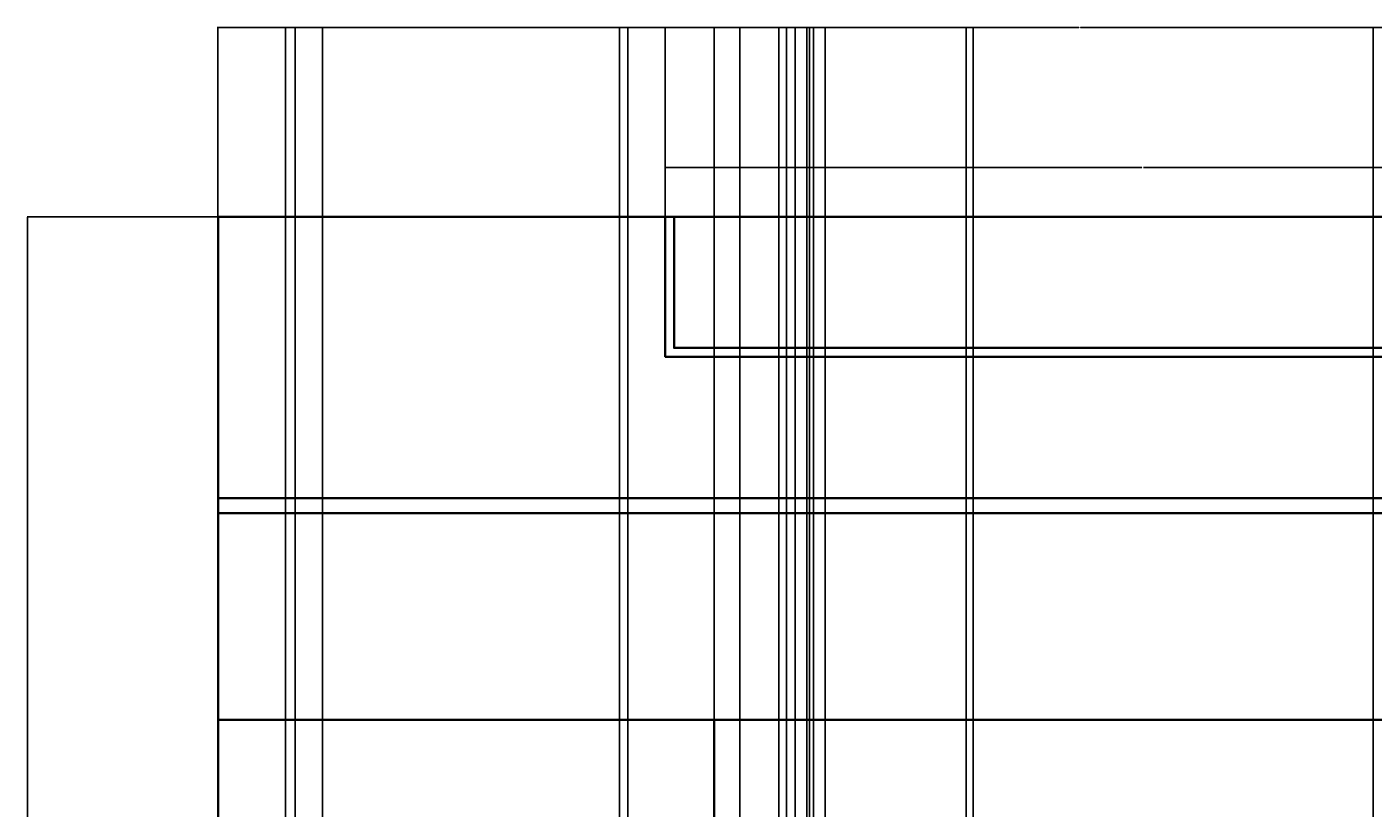
# Model space of a CAD drawing. Units: inches. Extents: x 1231 to 2151, y 481 to 2277.
# Tile 6 of 7: x 1231 to 1819, y 1935 to 2277. Entities that reach past the tile are written whole.
import ezdxf

# ---------------------------------------------------------------- set-up
doc = ezdxf.new("R2010")
doc.units = ezdxf.units.IN
doc.header["$MEASUREMENT"] = 0
doc.layers.add('A-ANNO-DIMS', color=2, linetype='Continuous', lineweight=18)
doc.layers.add('A-ELEV', color=7, linetype='Continuous', lineweight=35)
doc.styles.get("Standard").update_dxf_attribs({"font": 'arial.ttf'})
doc.dimstyles.get("Standard").update_dxf_attribs({"dimtxt": 0.18, "dimasz": 0.18, "dimexe": 0.18, "dimexo": 0.0625, "dimgap": 0.09, "dimtad": 0, "dimtih": 1, "dimtoh": 1, "dimdec": 0, "dimzin": 0, "dimdsep": 46, "dimlunit": 3, "dimtxsty": 'Standard', "dimcen": 0.09, "dimadec": 0, "dimazin": 0, "dimtfac": 1, "dimtdec": 0, "dimtofl": 0, "dimtmove": 0, "dimatfit": 3, "dimfxl": 1, "dimtolj": 1, "dimtzin": 0, "dimarcsym": 0})

# ---------------------------------------------------------------- blocks, each defined once
blk = doc.blocks.new('*D2')
at = {"layer": 'A-ANNO-DIMS', "color": 0, "lineweight": -2, "transparency": 16777216}
for p, q in [((1314.18, 2193.78), (1230.78, 2193.78)), ((1230.96, 2193.6), (1230.96, 1378.92)), ((1230.96, 563.87), (1230.96, 1378.55)), ((1314.18, 563.69), (1230.78, 563.69))]:
    blk.add_line(p, q, dxfattribs=at)
at = {"layer": 'A-ANNO-DIMS', "color": 0, "transparency": 16777216}
for points in [[(1230.93, 2193.6), (1230.99, 2193.6), (1230.96, 2193.78)], [(1230.93, 563.87), (1230.99, 563.87), (1230.96, 563.69)]]:
    blk.add_solid(points, dxfattribs=at)
at = {"layer": 'Defpoints', "color": 0, "transparency": 16777216}
for p in [(1230.96, 2193.78), (1314.24, 2193.78), (1314.24, 563.69)]:
    blk.add_point(p, dxfattribs=at)
at = {"layer": 'A-ANNO-DIMS', "color": 0, "transparency": 16777216, "insert": (1230.96, 1378.74), "char_height": 0.18, "attachment_point": 5}
blk.add_mtext('\\A1;1630', dxfattribs=at)
blk = doc.blocks.new('*D15')
at = {"layer": 'A-ANNO-DIMS', "color": 0, "lineweight": -2, "transparency": 16777216}
for p, q in [((1314.24, 1475.61), (1314.24, 2276.71)), ((1314.42, 2276.53), (1328.56, 2276.53)), ((1343.64, 2276.53), (1329.49, 2276.53)), ((1343.82, 1512.24), (1343.82, 2276.71))]:
    blk.add_line(p, q, dxfattribs=at)
at = {"layer": 'A-ANNO-DIMS', "color": 0, "transparency": 16777216}
for points in [[(1314.42, 2276.56), (1314.42, 2276.5), (1314.24, 2276.53)], [(1343.64, 2276.56), (1343.64, 2276.5), (1343.82, 2276.53)]]:
    blk.add_solid(points, dxfattribs=at)
at = {"layer": 'Defpoints', "color": 0, "transparency": 16777216}
for p in [(1343.82, 2276.53), (1343.82, 1512.17), (1314.24, 1475.54)]:
    blk.add_point(p, dxfattribs=at)
at = {"layer": 'A-ANNO-DIMS', "color": 0, "transparency": 16777216, "insert": (1329.03, 2276.53), "char_height": 0.18, "attachment_point": 5}
blk.add_mtext('\\A1;29.575', dxfattribs=at)
blk = doc.blocks.new('*D16')
at = {"layer": 'A-ANNO-DIMS', "color": 0, "lineweight": -2, "transparency": 16777216}
for p, q in [((1343.82, 1512.24), (1343.82, 2276.71)), ((1344, 2276.53), (1418.14, 2276.53)), ((1493.2, 2276.53), (1419.06, 2276.53)), ((1493.38, 1512.24), (1493.38, 2276.71))]:
    blk.add_line(p, q, dxfattribs=at)
at = {"layer": 'A-ANNO-DIMS', "color": 0, "transparency": 16777216}
for points in [[(1344, 2276.56), (1344, 2276.5), (1343.82, 2276.53)], [(1493.2, 2276.56), (1493.2, 2276.5), (1493.38, 2276.53)]]:
    blk.add_solid(points, dxfattribs=at)
at = {"layer": 'Defpoints', "color": 0, "transparency": 16777216}
for p in [(1493.38, 2276.53), (1343.82, 1512.17), (1493.38, 1512.17)]:
    blk.add_point(p, dxfattribs=at)
at = {"layer": 'A-ANNO-DIMS', "color": 0, "transparency": 16777216, "insert": (1418.6, 2276.53), "char_height": 0.18, "attachment_point": 5}
blk.add_mtext('\\A1;149.57', dxfattribs=at)
blk = doc.blocks.new('*D17')
at = {"layer": 'A-ANNO-DIMS', "color": 0, "lineweight": -2, "transparency": 16777216}
for p, q in [((1493.38, 1512.24), (1493.38, 2276.71)), ((1493.56, 2276.53), (1527.71, 2276.53)), ((1562.61, 2276.53), (1528.46, 2276.53)), ((1562.79, 1475.61), (1562.79, 2276.71))]:
    blk.add_line(p, q, dxfattribs=at)
at = {"layer": 'A-ANNO-DIMS', "color": 0, "transparency": 16777216}
for points in [[(1493.56, 2276.56), (1493.56, 2276.5), (1493.38, 2276.53)], [(1562.61, 2276.56), (1562.61, 2276.5), (1562.79, 2276.53)]]:
    blk.add_solid(points, dxfattribs=at)
at = {"layer": 'Defpoints', "color": 0, "transparency": 16777216}
for p in [(1562.79, 2276.53), (1493.38, 1512.17), (1562.79, 1475.54)]:
    blk.add_point(p, dxfattribs=at)
at = {"layer": 'A-ANNO-DIMS', "color": 0, "transparency": 16777216, "insert": (1528.09, 2276.53), "char_height": 0.18, "attachment_point": 5}
blk.add_mtext('\\A1;69.41', dxfattribs=at)
blk = doc.blocks.new('*D18')
at = {"layer": 'A-ANNO-DIMS', "color": 0, "lineweight": -2, "transparency": 16777216}
for p, q in [((1562.79, 1914.62), (1562.79, 2276.71)), ((1562.97, 2276.53), (1690.65, 2276.53)), ((1819.13, 2276.53), (1691.45, 2276.53)), ((1819.31, 1914.62), (1819.31, 2276.71))]:
    blk.add_line(p, q, dxfattribs=at)
at = {"layer": 'A-ANNO-DIMS', "color": 0, "transparency": 16777216}
for points in [[(1562.97, 2276.56), (1562.97, 2276.5), (1562.79, 2276.53)], [(1819.13, 2276.56), (1819.13, 2276.5), (1819.31, 2276.53)]]:
    blk.add_solid(points, dxfattribs=at)
at = {"layer": 'Defpoints', "color": 0, "transparency": 16777216}
for p in [(1819.31, 2276.53), (1562.79, 1914.56), (1819.31, 1914.56)]:
    blk.add_point(p, dxfattribs=at)
at = {"layer": 'A-ANNO-DIMS', "color": 0, "transparency": 16777216, "insert": (1691.05, 2276.53), "char_height": 0.18, "attachment_point": 5}
blk.add_mtext('\\A1;256.5', dxfattribs=at)
blk = doc.blocks.new('*D22')
at = {"layer": 'A-ANNO-DIMS', "color": 0, "lineweight": -2, "transparency": 16777216}
for p, q in [((1314.24, 1973.95), (1314.24, 2276.71)), ((1314.42, 2276.53), (1422.26, 2276.53)), ((1531.03, 2276.53), (1423.19, 2276.53)), ((1531.21, 1973.95), (1531.21, 2276.71))]:
    blk.add_line(p, q, dxfattribs=at)
at = {"layer": 'A-ANNO-DIMS', "color": 0, "transparency": 16777216}
for points in [[(1314.42, 2276.56), (1314.42, 2276.5), (1314.24, 2276.53)], [(1531.03, 2276.56), (1531.03, 2276.5), (1531.21, 2276.53)]]:
    blk.add_solid(points, dxfattribs=at)
at = {"layer": 'Defpoints', "color": 0, "transparency": 16777216}
for p in [(1531.21, 2276.53), (1314.24, 1973.89), (1531.21, 1973.89)]:
    blk.add_point(p, dxfattribs=at)
at = {"layer": 'A-ANNO-DIMS', "color": 0, "transparency": 16777216, "insert": (1422.73, 2276.53), "char_height": 0.18, "attachment_point": 5}
blk.add_mtext('\\A1;216.97', dxfattribs=at)
blk = doc.blocks.new('*D23')
at = {"layer": 'A-ANNO-DIMS', "color": 0, "lineweight": -2, "transparency": 16777216}
for p, q in [((1531.21, 1973.95), (1531.21, 2276.71)), ((1531.39, 2276.53), (1690.57, 2276.53)), ((1850.54, 2276.53), (1691.36, 2276.53)), ((1850.72, 1973.95), (1850.72, 2276.71))]:
    blk.add_line(p, q, dxfattribs=at)
at = {"layer": 'A-ANNO-DIMS', "color": 0, "transparency": 16777216}
for points in [[(1531.39, 2276.56), (1531.39, 2276.5), (1531.21, 2276.53)], [(1850.54, 2276.56), (1850.54, 2276.5), (1850.72, 2276.53)]]:
    blk.add_solid(points, dxfattribs=at)
at = {"layer": 'Defpoints', "color": 0, "transparency": 16777216}
for p in [(1850.72, 2276.53), (1531.21, 1973.89), (1850.72, 1973.89)]:
    blk.add_point(p, dxfattribs=at)
at = {"layer": 'A-ANNO-DIMS', "color": 0, "transparency": 16777216, "insert": (1690.96, 2276.53), "char_height": 0.18, "attachment_point": 5}
blk.add_mtext('\\A1;319.5', dxfattribs=at)
blk = doc.blocks.new('*D25')
at = {"layer": 'A-ANNO-DIMS', "color": 0, "lineweight": -2, "transparency": 16777216}
for p, q in [((1314.24, 2193.84), (1314.24, 2276.71)), ((1314.42, 2276.53), (1411.56, 2276.53)), ((1509.61, 2276.53), (1412.47, 2276.53)), ((1509.79, 2193.84), (1509.79, 2276.71))]:
    blk.add_line(p, q, dxfattribs=at)
at = {"layer": 'A-ANNO-DIMS', "color": 0, "transparency": 16777216}
for points in [[(1314.42, 2276.56), (1314.42, 2276.5), (1314.24, 2276.53)], [(1509.61, 2276.56), (1509.61, 2276.5), (1509.79, 2276.53)]]:
    blk.add_solid(points, dxfattribs=at)
at = {"layer": 'Defpoints', "color": 0, "transparency": 16777216}
for p in [(1509.79, 2276.53), (1314.24, 2193.78), (1509.79, 2193.78)]:
    blk.add_point(p, dxfattribs=at)
at = {"layer": 'A-ANNO-DIMS', "color": 0, "transparency": 16777216, "insert": (1412.02, 2276.53), "char_height": 0.18, "attachment_point": 5}
blk.add_mtext('\\A1;195.55', dxfattribs=at)
blk = doc.blocks.new('*D26')
at = {"layer": 'A-ANNO-DIMS', "color": 0, "lineweight": -2, "transparency": 16777216}
for p, q in [((1509.79, 2132.61), (1509.79, 2215.48)), ((1509.97, 2215.3), (1718.14, 2215.3)), ((1927.1, 2215.3), (1718.93, 2215.3)), ((1927.28, 2132.61), (1927.28, 2215.48))]:
    blk.add_line(p, q, dxfattribs=at)
at = {"layer": 'A-ANNO-DIMS', "color": 0, "transparency": 16777216}
for points in [[(1509.97, 2215.33), (1509.97, 2215.27), (1509.79, 2215.3)], [(1927.1, 2215.33), (1927.1, 2215.27), (1927.28, 2215.3)]]:
    blk.add_solid(points, dxfattribs=at)
at = {"layer": 'Defpoints', "color": 0, "transparency": 16777216}
for p in [(1927.28, 2215.3), (1509.79, 2132.55), (1927.28, 2132.55)]:
    blk.add_point(p, dxfattribs=at)
at = {"layer": 'A-ANNO-DIMS', "color": 0, "transparency": 16777216, "insert": (1718.53, 2215.3), "char_height": 0.18, "attachment_point": 5}
blk.add_mtext('\\A1;417.5', dxfattribs=at)
blk = doc.blocks.new('*D32')
at = {"layer": 'A-ANNO-DIMS', "color": 0, "lineweight": -2, "transparency": 16777216}
for p, q in [((1314.24, 1043.75), (1314.24, 2276.71)), ((1314.42, 2276.53), (1336.68, 2276.53)), ((1359.73, 2276.53), (1337.47, 2276.53)), ((1359.91, 1037.75), (1359.91, 2276.71))]:
    blk.add_line(p, q, dxfattribs=at)
at = {"layer": 'A-ANNO-DIMS', "color": 0, "transparency": 16777216}
for points in [[(1314.42, 2276.56), (1314.42, 2276.5), (1314.24, 2276.53)], [(1359.73, 2276.56), (1359.73, 2276.5), (1359.91, 2276.53)]]:
    blk.add_solid(points, dxfattribs=at)
at = {"layer": 'Defpoints', "color": 0, "transparency": 16777216}
for p in [(1359.91, 2276.53), (1314.24, 1043.69), (1359.91, 1037.69)]:
    blk.add_point(p, dxfattribs=at)
at = {"layer": 'A-ANNO-DIMS', "color": 0, "transparency": 16777216, "insert": (1337.07, 2276.53), "char_height": 0.18, "attachment_point": 5}
blk.add_mtext('\\A1;45.67', dxfattribs=at)
blk = doc.blocks.new('*D33')
at = {"layer": 'A-ANNO-DIMS', "color": 0, "lineweight": -2, "transparency": 16777216}
for p, q in [((1359.91, 1037.75), (1359.91, 2276.71)), ((1360.09, 2276.53), (1424.43, 2276.53)), ((1489.68, 2276.53), (1425.34, 2276.53)), ((1489.86, 1037.75), (1489.86, 2276.71))]:
    blk.add_line(p, q, dxfattribs=at)
at = {"layer": 'A-ANNO-DIMS', "color": 0, "transparency": 16777216}
for points in [[(1360.09, 2276.56), (1360.09, 2276.5), (1359.91, 2276.53)], [(1489.68, 2276.56), (1489.68, 2276.5), (1489.86, 2276.53)]]:
    blk.add_solid(points, dxfattribs=at)
at = {"layer": 'Defpoints', "color": 0, "transparency": 16777216}
for p in [(1489.86, 2276.53), (1359.91, 1037.69), (1489.86, 1037.69)]:
    blk.add_point(p, dxfattribs=at)
at = {"layer": 'A-ANNO-DIMS', "color": 0, "transparency": 16777216, "insert": (1424.88, 2276.53), "char_height": 0.18, "attachment_point": 5}
blk.add_mtext('\\A1;129.95', dxfattribs=at)
blk = doc.blocks.new('*D34')
at = {"layer": 'A-ANNO-DIMS', "color": 0, "lineweight": -2, "transparency": 16777216}
for p, q in [((1489.86, 1037.75), (1489.86, 2276.71)), ((1490.04, 2276.53), (1515.72, 2276.53)), ((1542.2, 2276.53), (1516.51, 2276.53)), ((1542.38, 1043.75), (1542.38, 2276.71))]:
    blk.add_line(p, q, dxfattribs=at)
at = {"layer": 'A-ANNO-DIMS', "color": 0, "transparency": 16777216}
for points in [[(1490.04, 2276.56), (1490.04, 2276.5), (1489.86, 2276.53)], [(1542.2, 2276.56), (1542.2, 2276.5), (1542.38, 2276.53)]]:
    blk.add_solid(points, dxfattribs=at)
at = {"layer": 'Defpoints', "color": 0, "transparency": 16777216}
for p in [(1542.38, 2276.53), (1542.38, 1043.69), (1489.86, 1037.69)]:
    blk.add_point(p, dxfattribs=at)
at = {"layer": 'A-ANNO-DIMS', "color": 0, "transparency": 16777216, "insert": (1516.12, 2276.53), "char_height": 0.18, "attachment_point": 5}
blk.add_mtext('\\A1;52.52', dxfattribs=at)
blk = doc.blocks.new('*D35')
at = {"layer": 'A-ANNO-DIMS', "color": 0, "lineweight": -2, "transparency": 16777216}
for p, q in [((1542.38, 1043.75), (1542.38, 2276.71)), ((1542.56, 2276.53), (1556.6, 2276.53)), ((1571.58, 2276.53), (1557.53, 2276.53)), ((1571.76, 1043.75), (1571.76, 2276.71))]:
    blk.add_line(p, q, dxfattribs=at)
at = {"layer": 'A-ANNO-DIMS', "color": 0, "transparency": 16777216}
for points in [[(1542.56, 2276.56), (1542.56, 2276.5), (1542.38, 2276.53)], [(1571.58, 2276.56), (1571.58, 2276.5), (1571.76, 2276.53)]]:
    blk.add_solid(points, dxfattribs=at)
at = {"layer": 'Defpoints', "color": 0, "transparency": 16777216}
for p in [(1571.76, 2276.53), (1542.38, 1043.69), (1571.76, 1043.69)]:
    blk.add_point(p, dxfattribs=at)
at = {"layer": 'A-ANNO-DIMS', "color": 0, "transparency": 16777216, "insert": (1557.07, 2276.53), "char_height": 0.18, "attachment_point": 5}
blk.add_mtext('\\A1;29.385', dxfattribs=at)
blk = doc.blocks.new('*D36')
at = {"layer": 'A-ANNO-DIMS', "color": 0, "lineweight": -2, "transparency": 16777216}
for p, q in [((1571.76, 1043.75), (1571.76, 2276.71)), ((1571.94, 2276.53), (1575.38, 2276.53)), ((1579.61, 2276.53), (1576.17, 2276.53)), ((1579.79, 1032.87), (1579.79, 2276.71))]:
    blk.add_line(p, q, dxfattribs=at)
at = {"layer": 'A-ANNO-DIMS', "color": 0, "transparency": 16777216}
for points in [[(1571.94, 2276.56), (1571.94, 2276.5), (1571.76, 2276.53)], [(1579.61, 2276.56), (1579.61, 2276.5), (1579.79, 2276.53)]]:
    blk.add_solid(points, dxfattribs=at)
at = {"layer": 'Defpoints', "color": 0, "transparency": 16777216}
for p in [(1579.79, 2276.53), (1571.76, 1043.69), (1579.79, 1032.81)]:
    blk.add_point(p, dxfattribs=at)
at = {"layer": 'A-ANNO-DIMS', "color": 0, "transparency": 16777216, "insert": (1575.78, 2276.53), "char_height": 0.18, "attachment_point": 5}
blk.add_mtext('\\A1;8.033', dxfattribs=at)
blk = doc.blocks.new('*D50')
at = {"layer": 'A-ANNO-DIMS', "color": 0, "lineweight": -2, "transparency": 16777216}
for p, q in [((1542.38, 563.75), (1542.38, 2276.71)), ((1542.56, 2276.53), (1550.52, 2276.53)), ((1559.26, 2276.53), (1551.3, 2276.53)), ((1559.44, 576.65), (1559.44, 2276.71))]:
    blk.add_line(p, q, dxfattribs=at)
at = {"layer": 'A-ANNO-DIMS', "color": 0, "transparency": 16777216}
for points in [[(1542.56, 2276.56), (1542.56, 2276.5), (1542.38, 2276.53)], [(1559.26, 2276.56), (1559.26, 2276.5), (1559.44, 2276.53)]]:
    blk.add_solid(points, dxfattribs=at)
at = {"layer": 'Defpoints', "color": 0, "transparency": 16777216}
for p in [(1559.44, 2276.53), (1559.44, 576.59), (1542.38, 563.69)]:
    blk.add_point(p, dxfattribs=at)
at = {"layer": 'A-ANNO-DIMS', "color": 0, "transparency": 16777216, "insert": (1550.91, 2276.53), "char_height": 0.18, "attachment_point": 5}
blk.add_mtext('\\A1;17.07', dxfattribs=at)
blk = doc.blocks.new('*D58')
at = {"layer": 'A-ANNO-DIMS', "color": 0, "lineweight": -2, "transparency": 16777216}
for p, q in [((1314.24, 1475.61), (1314.24, 2276.71)), ((1314.42, 2276.53), (1330.74, 2276.53)), ((1347.85, 2276.53), (1331.53, 2276.53)), ((1348.03, 1451.84), (1348.03, 2276.71))]:
    blk.add_line(p, q, dxfattribs=at)
at = {"layer": 'A-ANNO-DIMS', "color": 0, "transparency": 16777216}
for points in [[(1314.42, 2276.56), (1314.42, 2276.5), (1314.24, 2276.53)], [(1347.85, 2276.56), (1347.85, 2276.5), (1348.03, 2276.53)]]:
    blk.add_solid(points, dxfattribs=at)
at = {"layer": 'Defpoints', "color": 0, "transparency": 16777216}
for p in [(1348.03, 2276.53), (1314.24, 1475.54), (1348.03, 1451.77)]:
    blk.add_point(p, dxfattribs=at)
at = {"layer": 'A-ANNO-DIMS', "color": 0, "transparency": 16777216, "insert": (1331.14, 2276.53), "char_height": 0.18, "attachment_point": 5}
blk.add_mtext('\\A1;33.79', dxfattribs=at)
blk = doc.blocks.new('*D94')
at = {"layer": 'A-ANNO-DIMS', "color": 0, "lineweight": -2, "transparency": 16777216}
for p, q in [((1566.56, 1479.38), (1566.56, 2276.71)), ((1566.74, 2276.53), (1570.19, 2276.53)), ((1574.42, 2276.53), (1570.98, 2276.53)), ((1574.6, 1494.2), (1574.6, 2276.71))]:
    blk.add_line(p, q, dxfattribs=at)
at = {"layer": 'A-ANNO-DIMS', "color": 0, "transparency": 16777216}
for points in [[(1566.74, 2276.56), (1566.74, 2276.5), (1566.56, 2276.53)], [(1574.42, 2276.56), (1574.42, 2276.5), (1574.6, 2276.53)]]:
    blk.add_solid(points, dxfattribs=at)
at = {"layer": 'Defpoints', "color": 0, "transparency": 16777216}
for p in [(1574.6, 2276.53), (1574.6, 1494.13), (1566.56, 1479.32)]:
    blk.add_point(p, dxfattribs=at)
at = {"layer": 'A-ANNO-DIMS', "color": 0, "transparency": 16777216, "insert": (1570.58, 2276.53), "char_height": 0.18, "attachment_point": 5}
blk.add_mtext('\\A1;8.042', dxfattribs=at)
blk = doc.blocks.new('*D95')
at = {"layer": 'A-ANNO-DIMS', "color": 0, "lineweight": -2, "transparency": 16777216}
for p, q in [((1574.6, 1494.2), (1574.6, 2276.71)), ((1574.78, 2276.53), (1607.58, 2276.53)), ((1641.16, 2276.53), (1608.37, 2276.53)), ((1641.34, 1494.2), (1641.34, 2276.71))]:
    blk.add_line(p, q, dxfattribs=at)
at = {"layer": 'A-ANNO-DIMS', "color": 0, "transparency": 16777216}
for points in [[(1574.78, 2276.56), (1574.78, 2276.5), (1574.6, 2276.53)], [(1641.16, 2276.56), (1641.16, 2276.5), (1641.34, 2276.53)]]:
    blk.add_solid(points, dxfattribs=at)
at = {"layer": 'Defpoints', "color": 0, "transparency": 16777216}
for p in [(1641.34, 2276.53), (1574.6, 1494.13), (1641.34, 1494.13)]:
    blk.add_point(p, dxfattribs=at)
at = {"layer": 'A-ANNO-DIMS', "color": 0, "transparency": 16777216, "insert": (1607.97, 2276.53), "char_height": 0.18, "attachment_point": 5}
blk.add_mtext('\\A1;66.74', dxfattribs=at)
blk = doc.blocks.new('*D96')
at = {"layer": 'A-ANNO-DIMS', "color": 0, "lineweight": -2, "transparency": 16777216}
for p, q in [((1572.87, 1828.31), (1572.87, 2276.71)), ((1573.05, 2276.53), (1608.26, 2276.53)), ((1644.26, 2276.53), (1609.05, 2276.53)), ((1644.44, 1828.31), (1644.44, 2276.71))]:
    blk.add_line(p, q, dxfattribs=at)
at = {"layer": 'A-ANNO-DIMS', "color": 0, "transparency": 16777216}
for points in [[(1573.05, 2276.56), (1573.05, 2276.5), (1572.87, 2276.53)], [(1644.26, 2276.56), (1644.26, 2276.5), (1644.44, 2276.53)]]:
    blk.add_solid(points, dxfattribs=at)
at = {"layer": 'Defpoints', "color": 0, "transparency": 16777216}
for p in [(1644.44, 2276.53), (1572.87, 1828.25), (1644.44, 1828.25)]:
    blk.add_point(p, dxfattribs=at)
at = {"layer": 'A-ANNO-DIMS', "color": 0, "transparency": 16777216, "insert": (1608.65, 2276.53), "char_height": 0.18, "attachment_point": 5}
blk.add_mtext('\\A1;71.57', dxfattribs=at)

msp = doc.modelspace()

# ---------------------------------------------------------------- linework, layer by layer
at = {"layer": 'A-ELEV'}
for p, q in [((1314.2408, 1475.5441), (1314.2408, 2193.7789)), ((2067.6855, 2193.7789), (1314.2408, 2193.7789)), ((2067.6855, 2070.8244), (1314.2408, 2070.8244)), ((2067.6855, 2064.2116), (1314.2408, 2064.2116)), ((2067.6855, 1973.8854), (1314.2408, 1973.8854)), ((1531.2103, 1475.5441), (1531.2103, 1973.8854))]:
    msp.add_line(p, q, dxfattribs=at)
msp.add_lwpolyline([(1927.277, 2193.7789), (1927.277, 2132.5472), (1509.7902, 2132.5472), (1509.7902, 2193.7789)], dxfattribs=at)
msp.add_lwpolyline([(1513.6622, 2193.7789), (1923.405, 2193.7789), (1923.405, 2136.4192), (1513.6622, 2136.4192)], close=True, dxfattribs=at)

# ---------------------------------------------------------------- dimensions: what is measured, and where the dimension line sits
at = {"layer": 'A-ANNO-DIMS'}
for base, p1, p2, override, picture, middle in [((1343.8157, 2276.5289), (1314.2408, 1475.5441), (1343.8157, 1512.1749), {"dimdec": 3, "dimlfac": 1, "dimrnd": 0, "dimzin": 0, "dimdsep": 46, "dimlunit": 2}, '*D15', (1329.0282, 2276.5289)), ((1531.2103, 2276.5289), (1314.2408, 1973.8854), (1531.2103, 1973.8854), {"dimdec": 2, "dimlfac": 1, "dimrnd": 0, "dimzin": 0, "dimdsep": 46, "dimlunit": 2}, '*D22', (1422.7256, 2276.5289)), ((1509.7902, 2276.5289), (1314.2408, 2193.7789), (1509.7902, 2193.7789), {"dimdec": 2, "dimlfac": 1, "dimrnd": 0, "dimzin": 0, "dimdsep": 46, "dimlunit": 2}, '*D25', (1412.0155, 2276.5289)), ((1359.9075, 2276.5289), (1314.2408, 1043.6912), (1359.9075, 1037.6872), {"dimdec": 2, "dimlfac": 1, "dimrnd": 0, "dimzin": 0, "dimdsep": 46, "dimlunit": 2}, '*D32', (1337.0741, 2276.5289)), ((1348.0309, 2276.5289), (1314.2408, 1475.5441), (1348.0309, 1451.7741), {"dimdec": 2, "dimlfac": 1, "dimrnd": 0, "dimzin": 0, "dimdsep": 46, "dimlunit": 2}, '*D58', (1331.1358, 2276.5289)), ((1493.3841, 2276.5289), (1343.8157, 1512.1749), (1493.3841, 1512.1749), {"dimdec": 2, "dimlfac": 1, "dimrnd": 0, "dimzin": 0, "dimdsep": 46, "dimlunit": 2}, '*D16', (1418.5999, 2276.5289)), ((1489.8565, 2276.5289), (1359.9075, 1037.6872), (1489.8565, 1037.6872), {"dimdec": 2, "dimlfac": 1, "dimrnd": 0, "dimzin": 0, "dimdsep": 46, "dimlunit": 2}, '*D33', (1424.882, 2276.5289)), ((1542.3752, 2276.5289), (1489.8565, 1037.6872), (1542.3752, 1043.6912), {"dimdec": 2, "dimlfac": 1, "dimrnd": 0, "dimzin": 0, "dimdsep": 46, "dimlunit": 2}, '*D34', (1516.1158, 2276.5289)), ((1562.7916, 2276.5289), (1493.3841, 1512.1749), (1562.7916, 1475.5441), {"dimdec": 2, "dimlfac": 1, "dimrnd": 0, "dimzin": 0, "dimdsep": 46, "dimlunit": 2}, '*D17', (1528.0878, 2276.5289)), ((1850.716, 2276.5289), (1531.2103, 1973.8854), (1850.716, 1973.8854), {"dimdec": 1, "dimlfac": 1, "dimrnd": 0, "dimzin": 0, "dimdsep": 46, "dimlunit": 2}, '*D23', (1690.9632, 2276.5289)), ((1571.76, 2276.5289), (1542.3752, 1043.6912), (1571.76, 1043.6912), {"dimdec": 3, "dimlfac": 1, "dimrnd": 0, "dimzin": 0, "dimdsep": 46, "dimlunit": 2}, '*D35', (1557.0676, 2276.5289)), ((1559.4446, 2276.5289), (1542.3752, 563.6912), (1559.4446, 576.5889), {"dimdec": 2, "dimlfac": 1, "dimrnd": 0, "dimzin": 0, "dimdsep": 46, "dimlunit": 2}, '*D50', (1550.9099, 2276.5289)), ((1819.3087, 2276.5289), (1562.7916, 1914.557), (1819.3087, 1914.557), {"dimdec": 1, "dimlfac": 1, "dimrnd": 0, "dimzin": 0, "dimdsep": 46, "dimlunit": 2}, '*D18', (1691.0501, 2276.5289)), ((1574.6049, 2276.5289), (1566.5626, 1479.3152), (1574.6049, 1494.1329), {"dimdec": 3, "dimlfac": 1, "dimrnd": 0, "dimzin": 0, "dimdsep": 46, "dimlunit": 2}, '*D94', (1570.5838, 2276.5289)), ((1579.7928, 2276.5289), (1571.76, 1043.6912), (1579.7928, 1032.8111), {"dimdec": 3, "dimlfac": 1, "dimrnd": 0, "dimzin": 0, "dimdsep": 46, "dimlunit": 2}, '*D36', (1575.7764, 2276.5289)), ((1644.4374, 2276.5289), (1572.8669, 1828.2487), (1644.4374, 1828.2487), {"dimdec": 2, "dimlfac": 1, "dimrnd": 0, "dimzin": 0, "dimdsep": 46, "dimlunit": 2}, '*D96', (1608.6522, 2276.5289)), ((1641.3412, 2276.5289), (1574.6049, 1494.1329), (1641.3412, 1494.1329), {"dimdec": 2, "dimlfac": 1, "dimrnd": 0, "dimzin": 0, "dimdsep": 46, "dimlunit": 2}, '*D95', (1607.973, 2276.5289)), ((1927.277, 2215.2972), (1509.7902, 2132.5472), (1927.277, 2132.5472), {"dimdec": 1, "dimlfac": 1, "dimrnd": 0, "dimzin": 0, "dimdsep": 46, "dimlunit": 2}, '*D26', (1718.5336, 2215.2972))]:
    dim = msp.add_linear_dim(base=base, p1=p1, p2=p2, dimstyle='Standard', override=override, dxfattribs=at)
    dim.commit()
    dim.dimension.update_dxf_attribs({"geometry": picture, "text_midpoint": middle})
dim = msp.add_linear_dim(base=(1230.9629, 2193.7789), p1=(1314.2408, 563.6912), p2=(1314.2408, 2193.7789), angle=90, dimstyle='Standard', override={"dimdec": 0, "dimlfac": 1, "dimrnd": 0, "dimzin": 0, "dimdsep": 46, "dimlunit": 2}, dxfattribs=at)
dim.commit()
dim.dimension.update_dxf_attribs({"geometry": '*D2', "text_midpoint": (1230.9629, 1378.7351)})

doc.saveas('drawing.dxf')
